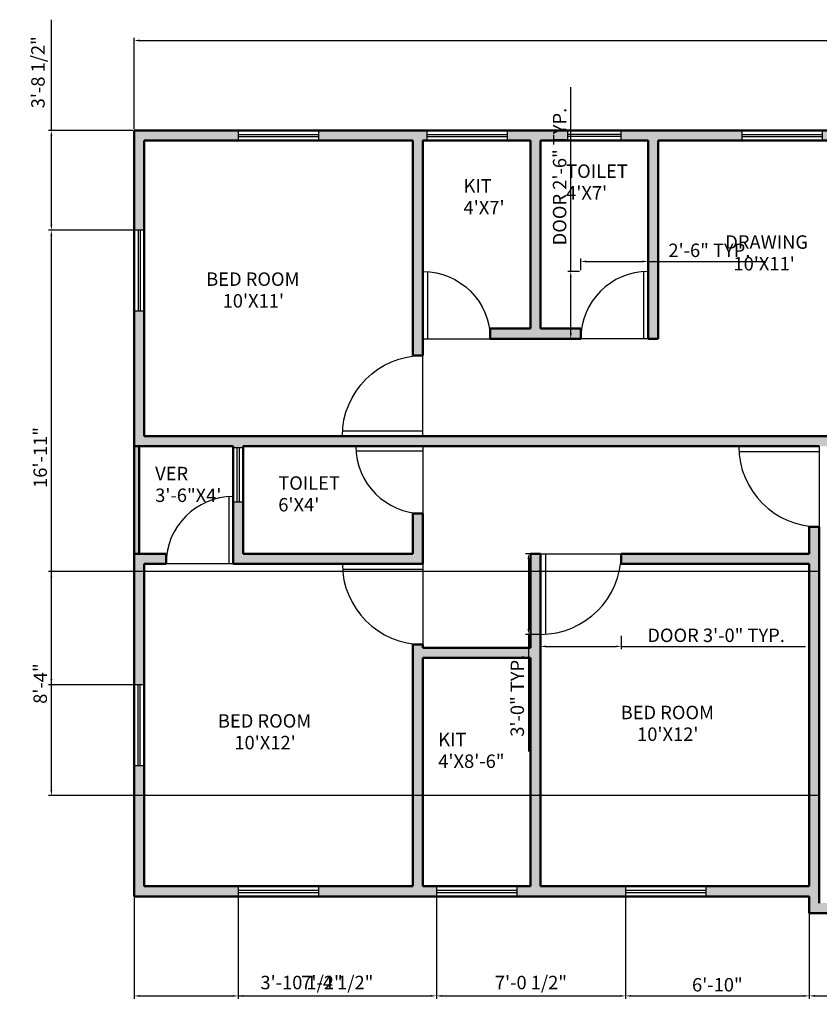
# Model space of a CAD drawing. Units: inches. Extents: x 1931 to 2735, y 1903 to 2370.
# Tile 1 of 2: x 1931 to 2288, y 1903 to 2343. Entities that reach past the tile are written whole.
import ezdxf

# ---------------------------------------------------------------- set-up
doc = ezdxf.new("R2010")
doc.units = ezdxf.units.IN
doc.header["$LTSCALE"] = 0.5
for name, color, linetype, lineweight in [('A-ANNO-DIMS', 93, 'Continuous', 18), ('A-AREA-IDEN', 93, 'Continuous', 25), ('DOORS', 121, 'Continuous', 25), ('WALLS', 231, 'Continuous', 50), ('WINDOWS', 200, 'Continuous', 25)]:
    doc.layers.add(name, color=color, linetype=linetype, lineweight=lineweight)
doc.layers.add('A-WALL-PATT', color=143, linetype='Continuous', lineweight=13, true_color=0x7aafdf)
doc.styles.get("Standard").update_dxf_attribs({"font": 'txt', "height": 6})
doc.dimstyles.new('ISO-25', dxfattribs={"dimtxt": 5, "dimasz": 2.5, "dimexe": 1.25, "dimexo": 0.625, "dimtad": 1, "dimlunit": 3, "dimtxsty": 'Standard', "dimcen": 2.5, "dimadec": 0, "dimazin": 0, "dimtfac": 1, "dimtmove": 0, "dimatfit": 3, "dimfxl": 1, "dimarcsym": 0})

# ---------------------------------------------------------------- blocks, each defined once
blk = doc.blocks.new('*D1')
at = {"layer": 'A-ANNO-DIMS', "color": 0, "lineweight": -2, "transparency": 16777216}
for p, q in [((1982.32, 2294.17), (1982.32, 2334.97)), ((2694.32, 2294.17), (2694.32, 2334.97)), ((1984.82, 2333.72), (2691.82, 2333.72))]:
    blk.add_line(p, q, dxfattribs=at)
at = {"layer": 'A-ANNO-DIMS', "color": 0, "lineweight": 100, "transparency": 16777216}
for points in [[(1984.82, 2334.14), (1984.82, 2333.3), (1982.32, 2333.72)], [(2691.82, 2334.14), (2691.82, 2333.3), (2694.32, 2333.72)]]:
    blk.add_solid(points, dxfattribs=at)
at = {"layer": 'Defpoints', "color": 0, "lineweight": 100, "transparency": 16777216}
for p in [(2694.32, 2333.72), (1982.32, 2293.55), (2694.32, 2293.55)]:
    blk.add_point(p, dxfattribs=at)
at = {"layer": 'A-ANNO-DIMS', "color": 0, "transparency": 16777216, "insert": (2338.32, 2337.92), "char_height": 6, "attachment_point": 5}
blk.add_mtext('59\'-4"', dxfattribs=at)
blk = doc.blocks.new('DOOR-SWING-36IN')
for p, q in [((0, 0), (0, 36)), ((35.92, 2.4), (0, 2.4)), ((36, 0), (0, 0))]:
    blk.add_line(p, q)
blk.add_arc((0, 0), 36, 0, 90)
blk = doc.blocks.new('DOOR-SWING-30IN')
for p, q in [((28, 29.93), (28, 0)), ((30, 30), (30, 0)), ((30, 0), (0, 0))]:
    blk.add_line(p, q)
blk.add_arc((30, 0), 30, 90, 180)
blk = doc.blocks.new('WINDOW-36IN')
for p, q in [((0, 36), (0, 0)), ((4.5, 36), (0, 36)), ((1.75, 36), (1.75, 0)), ((2.75, 36), (2.75, 0)), ((4.5, 0), (4.5, 36)), ((0, 0), (4.5, 0))]:
    blk.add_line(p, q)
blk = doc.blocks.new('WINDOW-24IN')
for p, q in [((24, 4.5), (0, 4.5)), ((0, 4.5), (0, 0)), ((24, 0), (24, 4.5)), ((24, 2.75), (0, 2.75)), ((24, 1.75), (0, 1.75)), ((0, 0), (24, 0))]:
    blk.add_line(p, q)
blk = doc.blocks.new('*D11')
at = {"layer": 'A-ANNO-DIMS', "color": 0, "lineweight": -2, "transparency": 16777216}
for p, q in [((2163.82, 2067.92), (2163.82, 2061.9)), ((2199.82, 2067.92), (2199.82, 2061.9)), ((2166.32, 2063.15), (2197.32, 2063.15)), ((2199.82, 2063.15), (2282.14, 2063.15))]:
    blk.add_line(p, q, dxfattribs=at)
at = {"layer": 'A-ANNO-DIMS', "color": 0, "lineweight": 100, "transparency": 16777216}
for points in [[(2166.32, 2063.56), (2166.32, 2062.73), (2163.82, 2063.15)], [(2197.32, 2063.56), (2197.32, 2062.73), (2199.82, 2063.15)]]:
    blk.add_solid(points, dxfattribs=at)
at = {"layer": 'Defpoints', "color": 0, "lineweight": 100, "transparency": 16777216}
for p in [(2163.82, 2068.55), (2199.82, 2068.55), (2199.82, 2063.15)]:
    blk.add_point(p, dxfattribs=at)
at = {"layer": 'A-ANNO-DIMS', "color": 0, "transparency": 16777216, "insert": (2242.23, 2067.34), "char_height": 6, "attachment_point": 5}
blk.add_mtext('DOOR 3\'-0" TYP.', dxfattribs=at)
blk = doc.blocks.new('*D12')
at = {"layer": 'A-ANNO-DIMS', "color": 0, "lineweight": -2, "transparency": 16777216}
for p, q in [((2163.19, 2104.55), (2157.17, 2104.55)), ((2158.42, 2102.05), (2158.42, 2071.05)), ((2163.19, 2068.55), (2157.17, 2068.55)), ((2158.42, 2068.55), (2158.42, 2016.22))]:
    blk.add_line(p, q, dxfattribs=at)
at = {"layer": 'A-ANNO-DIMS', "color": 0, "lineweight": 100, "transparency": 16777216}
for points in [[(2158, 2102.05), (2158.83, 2102.05), (2158.42, 2104.55)], [(2158, 2071.05), (2158.83, 2071.05), (2158.42, 2068.55)]]:
    blk.add_solid(points, dxfattribs=at)
at = {"layer": 'Defpoints', "color": 0, "lineweight": 100, "transparency": 16777216}
for p in [(2163.82, 2104.55), (2158.42, 2068.55), (2163.82, 2068.55)]:
    blk.add_point(p, dxfattribs=at)
at = {"layer": 'A-ANNO-DIMS', "color": 0, "transparency": 16777216, "insert": (2154.22, 2041.13), "char_height": 6, "attachment_point": 5, "rotation": 90}
blk.add_mtext('3\'-0" TYP.', dxfattribs=at)
blk = doc.blocks.new('*D13')
at = {"layer": 'A-ANNO-DIMS', "color": 0, "lineweight": -2, "transparency": 16777216}
for p, q in [((2177.32, 2230.55), (2177.32, 2312.87)), ((2181.19, 2230.55), (2176.07, 2230.55)), ((2177.32, 2203.05), (2177.32, 2228.05)), ((2181.19, 2200.55), (2176.07, 2200.55))]:
    blk.add_line(p, q, dxfattribs=at)
at = {"layer": 'A-ANNO-DIMS', "color": 0, "lineweight": 100, "transparency": 16777216}
for points in [[(2176.9, 2228.05), (2177.73, 2228.05), (2177.32, 2230.55)], [(2176.9, 2203.05), (2177.73, 2203.05), (2177.32, 2200.55)]]:
    blk.add_solid(points, dxfattribs=at)
at = {"layer": 'Defpoints', "color": 0, "lineweight": 100, "transparency": 16777216}
for p in [(2177.32, 2230.55), (2181.82, 2230.55), (2181.82, 2200.55)]:
    blk.add_point(p, dxfattribs=at)
at = {"layer": 'A-ANNO-DIMS', "color": 0, "transparency": 16777216, "insert": (2173.12, 2272.96), "char_height": 6, "attachment_point": 5, "rotation": 90}
blk.add_mtext('DOOR 2\'-6" TYP.', dxfattribs=at)
blk = doc.blocks.new('*D14')
at = {"layer": 'A-ANNO-DIMS', "color": 0, "lineweight": -2, "transparency": 16777216}
for p, q in [((2181.82, 2231.17), (2181.82, 2236.3)), ((2184.32, 2235.05), (2209.32, 2235.05)), ((2211.82, 2231.17), (2211.82, 2236.3)), ((2211.82, 2235.05), (2264.14, 2235.05))]:
    blk.add_line(p, q, dxfattribs=at)
at = {"layer": 'A-ANNO-DIMS', "color": 0, "lineweight": 100, "transparency": 16777216}
for points in [[(2184.32, 2235.46), (2184.32, 2234.63), (2181.82, 2235.05)], [(2209.32, 2235.46), (2209.32, 2234.63), (2211.82, 2235.05)]]:
    blk.add_solid(points, dxfattribs=at)
at = {"layer": 'Defpoints', "color": 0, "lineweight": 100, "transparency": 16777216}
for p in [(2211.82, 2235.05), (2181.82, 2230.55), (2211.82, 2230.55)]:
    blk.add_point(p, dxfattribs=at)
at = {"layer": 'A-ANNO-DIMS', "color": 0, "transparency": 16777216, "insert": (2239.23, 2239.24), "char_height": 6, "attachment_point": 5}
blk.add_mtext('2\'-6" TYP.', dxfattribs=at)
blk = doc.blocks.new('*D15')
at = {"layer": 'A-ANNO-DIMS', "color": 0, "lineweight": -2, "transparency": 16777216}
for p, q in [((1982.32, 1950.92), (1982.32, 1905.85)), ((2028.82, 1950.92), (2028.82, 1905.85)), ((1984.82, 1907.1), (2026.32, 1907.1)), ((2028.82, 1907.1), (2082.85, 1907.1))]:
    blk.add_line(p, q, dxfattribs=at)
at = {"layer": 'A-ANNO-DIMS', "color": 0, "lineweight": 100, "transparency": 16777216}
for points in [[(1984.82, 1907.51), (1984.82, 1906.68), (1982.32, 1907.1)], [(2026.32, 1907.51), (2026.32, 1906.68), (2028.82, 1907.1)]]:
    blk.add_solid(points, dxfattribs=at)
at = {"layer": 'Defpoints', "color": 0, "lineweight": 100, "transparency": 16777216}
for p in [(1982.32, 1951.55), (2028.82, 1951.55), (2028.82, 1907.1)]:
    blk.add_point(p, dxfattribs=at)
at = {"layer": 'A-ANNO-DIMS', "color": 0, "transparency": 16777216, "insert": (2057.09, 1912.29), "char_height": 6, "attachment_point": 5}
blk.add_mtext('3\'-10 1/2"', dxfattribs=at)
blk = doc.blocks.new('*D16')
at = {"layer": 'A-ANNO-DIMS', "color": 0, "lineweight": -2, "transparency": 16777216}
for p, q in [((2028.82, 1950.92), (2028.82, 1905.85)), ((2117.32, 1950.92), (2117.32, 1905.85)), ((2031.32, 1907.1), (2114.82, 1907.1))]:
    blk.add_line(p, q, dxfattribs=at)
at = {"layer": 'A-ANNO-DIMS', "color": 0, "lineweight": 100, "transparency": 16777216}
for points in [[(2031.32, 1907.51), (2031.32, 1906.68), (2028.82, 1907.1)], [(2114.82, 1907.51), (2114.82, 1906.68), (2117.32, 1907.1)]]:
    blk.add_solid(points, dxfattribs=at)
at = {"layer": 'Defpoints', "color": 0, "lineweight": 100, "transparency": 16777216}
for p in [(2028.82, 1951.55), (2117.32, 1951.55), (2117.32, 1907.1)]:
    blk.add_point(p, dxfattribs=at)
at = {"layer": 'A-ANNO-DIMS', "color": 0, "transparency": 16777216, "insert": (2073.07, 1912.29), "char_height": 6, "attachment_point": 5}
blk.add_mtext('7\'-4 1/2"', dxfattribs=at)
blk = doc.blocks.new('*D17')
at = {"layer": 'A-ANNO-DIMS', "color": 0, "lineweight": -2, "transparency": 16777216}
for p, q in [((2117.32, 1950.92), (2117.32, 1905.85)), ((2201.75, 1950.92), (2201.75, 1905.85)), ((2119.82, 1907.1), (2199.25, 1907.1))]:
    blk.add_line(p, q, dxfattribs=at)
at = {"layer": 'A-ANNO-DIMS', "color": 0, "lineweight": 100, "transparency": 16777216}
for points in [[(2119.82, 1907.51), (2119.82, 1906.68), (2117.32, 1907.1)], [(2199.25, 1907.51), (2199.25, 1906.68), (2201.75, 1907.1)]]:
    blk.add_solid(points, dxfattribs=at)
at = {"layer": 'Defpoints', "color": 0, "lineweight": 100, "transparency": 16777216}
for p in [(2117.32, 1951.55), (2201.75, 1951.55), (2201.75, 1907.1)]:
    blk.add_point(p, dxfattribs=at)
at = {"layer": 'A-ANNO-DIMS', "color": 0, "transparency": 16777216, "insert": (2159.53, 1912.29), "char_height": 6, "attachment_point": 5}
blk.add_mtext('7\'-0 1/2"', dxfattribs=at)
blk = doc.blocks.new('*D18')
at = {"layer": 'A-ANNO-DIMS', "color": 0, "lineweight": -2, "transparency": 16777216}
for p, q in [((2201.75, 1950.92), (2201.75, 1905.85)), ((2283.82, 1950.92), (2283.82, 1905.85)), ((2204.25, 1907.1), (2281.32, 1907.1))]:
    blk.add_line(p, q, dxfattribs=at)
at = {"layer": 'A-ANNO-DIMS', "color": 0, "lineweight": 100, "transparency": 16777216}
for points in [[(2204.25, 1907.51), (2204.25, 1906.68), (2201.75, 1907.1)], [(2281.32, 1907.51), (2281.32, 1906.68), (2283.82, 1907.1)]]:
    blk.add_solid(points, dxfattribs=at)
at = {"layer": 'Defpoints', "color": 0, "lineweight": 100, "transparency": 16777216}
for p in [(2201.75, 1951.55), (2283.82, 1951.55), (2283.82, 1907.1)]:
    blk.add_point(p, dxfattribs=at)
at = {"layer": 'A-ANNO-DIMS', "color": 0, "transparency": 16777216, "insert": (2242.78, 1911.29), "char_height": 6, "attachment_point": 5}
blk.add_mtext('6\'-10"', dxfattribs=at)
blk = doc.blocks.new('*D19')
at = {"layer": 'A-ANNO-DIMS', "color": 0, "lineweight": -2, "transparency": 16777216}
for p, q in [((2283.82, 1943.42), (2283.82, 1905.85)), ((2312.44, 1943.42), (2312.44, 1905.85)), ((2286.32, 1907.1), (2309.94, 1907.1)), ((2312.44, 1907.1), (2361.91, 1907.1))]:
    blk.add_line(p, q, dxfattribs=at)
at = {"layer": 'A-ANNO-DIMS', "color": 0, "lineweight": 100, "transparency": 16777216}
for points in [[(2286.32, 1907.51), (2286.32, 1906.68), (2283.82, 1907.1)], [(2309.94, 1907.51), (2309.94, 1906.68), (2312.44, 1907.1)]]:
    blk.add_solid(points, dxfattribs=at)
at = {"layer": 'Defpoints', "color": 0, "lineweight": 100, "transparency": 16777216}
for p in [(2283.82, 1944.05), (2312.44, 1944.05), (2312.44, 1907.1)]:
    blk.add_point(p, dxfattribs=at)
at = {"layer": 'A-ANNO-DIMS', "color": 0, "transparency": 16777216, "insert": (2338.42, 1912.29), "char_height": 6, "attachment_point": 5}
blk.add_mtext('2\'-4 1/2"', dxfattribs=at)
blk = doc.blocks.new('*D26')
at = {"layer": 'A-ANNO-DIMS', "color": 0, "lineweight": -2, "transparency": 16777216}
for p, q in [((2287.69, 2096.55), (1944.12, 2096.55)), ((1945.37, 1999.05), (1945.37, 2094.05)), ((2287.69, 1996.55), (1944.12, 1996.55))]:
    blk.add_line(p, q, dxfattribs=at)
at = {"layer": 'A-ANNO-DIMS', "color": 0, "lineweight": 100, "transparency": 16777216}
for points in [[(1944.95, 2094.05), (1945.78, 2094.05), (1945.37, 2096.55)], [(1944.95, 1999.05), (1945.78, 1999.05), (1945.37, 1996.55)]]:
    blk.add_solid(points, dxfattribs=at)
at = {"layer": 'Defpoints', "color": 0, "lineweight": 100, "transparency": 16777216}
for p in [(1945.37, 2096.55), (2288.32, 2096.55), (2288.32, 1996.55)]:
    blk.add_point(p, dxfattribs=at)
at = {"layer": 'A-ANNO-DIMS', "color": 0, "transparency": 16777216, "insert": (1941.17, 2046.55), "char_height": 6, "attachment_point": 5, "rotation": 90}
blk.add_mtext('8\'-4"', dxfattribs=at)
blk = doc.blocks.new('*D28')
at = {"layer": 'A-ANNO-DIMS', "color": 0, "lineweight": -2, "transparency": 16777216}
for p, q in [((1945.37, 2293.55), (1945.37, 2343.01)), ((1981.69, 2293.55), (1944.12, 2293.55)), ((1945.37, 2251.5), (1945.37, 2291.05)), ((1981.69, 2249), (1944.12, 2249))]:
    blk.add_line(p, q, dxfattribs=at)
at = {"layer": 'A-ANNO-DIMS', "color": 0, "lineweight": 100, "transparency": 16777216}
for points in [[(1944.95, 2291.05), (1945.78, 2291.05), (1945.37, 2293.55)], [(1944.95, 2251.5), (1945.78, 2251.5), (1945.37, 2249)]]:
    blk.add_solid(points, dxfattribs=at)
at = {"layer": 'Defpoints', "color": 0, "lineweight": 100, "transparency": 16777216}
for p in [(1945.37, 2293.55), (1982.32, 2293.55), (1982.32, 2249)]:
    blk.add_point(p, dxfattribs=at)
at = {"layer": 'A-ANNO-DIMS', "color": 0, "transparency": 16777216, "insert": (1940.17, 2319.53), "char_height": 6, "attachment_point": 5, "rotation": 90}
blk.add_mtext('3\'-8 1/2"', dxfattribs=at)
blk = doc.blocks.new('*D29')
at = {"layer": 'A-ANNO-DIMS', "color": 0, "lineweight": -2, "transparency": 16777216}
for p, q in [((1981.69, 2249), (1944.12, 2249)), ((1945.37, 2048.55), (1945.37, 2246.5)), ((1981.69, 2046.05), (1944.12, 2046.05))]:
    blk.add_line(p, q, dxfattribs=at)
at = {"layer": 'A-ANNO-DIMS', "color": 0, "lineweight": 100, "transparency": 16777216}
for points in [[(1944.95, 2246.5), (1945.78, 2246.5), (1945.37, 2249)], [(1944.95, 2048.55), (1945.78, 2048.55), (1945.37, 2046.05)]]:
    blk.add_solid(points, dxfattribs=at)
at = {"layer": 'Defpoints', "color": 0, "lineweight": 100, "transparency": 16777216}
for p in [(1945.37, 2249), (1982.32, 2249), (1982.32, 2046.05)]:
    blk.add_point(p, dxfattribs=at)
at = {"layer": 'A-ANNO-DIMS', "color": 0, "transparency": 16777216, "insert": (1941.17, 2147.52), "char_height": 6, "attachment_point": 5, "rotation": 90}
blk.add_mtext('16\'-11"', dxfattribs=at)

msp = doc.modelspace()

# ---------------------------------------------------------------- hatches: boundary and pattern name
at = {"layer": 'A-WALL-PATT'}
h = msp.add_hatch(color=256, dxfattribs=at)
h.dxf.hatch_style = 1
h.paths.add_polyline_path([(2028.817, 2293.545), (1982.317, 2293.545), (1982.317, 2249.002), (1986.817, 2249.002), (1986.817, 2289.045), (2028.817, 2289.045)])
h.paths.add_polyline_path([(2113.054, 2293.545), (2064.817, 2293.545), (2064.817, 2289.045), (2106.817, 2289.045), (2106.817, 2193.045), (2111.317, 2193.045), (2111.317, 2200.545), (2111.317, 2230.545), (2111.317, 2289.045), (2113.054, 2289.045)])
h.paths.add_polyline_path([(2175.817, 2293.545), (2149.054, 2293.545), (2149.054, 2289.045), (2159.317, 2289.045), (2159.317, 2205.045), (2141.317, 2205.045), (2141.317, 2200.545), (2181.817, 2200.545), (2181.817, 2205.045), (2163.817, 2205.045), (2163.817, 2289.045), (2175.817, 2289.045)])
h.paths.add_polyline_path([(2253.691, 2293.545), (2199.817, 2293.545), (2199.817, 2289.045), (2211.817, 2289.045), (2211.817, 2200.545), (2216.317, 2200.545), (2216.317, 2289.045), (2253.691, 2289.045)])
h.paths.add_polyline_path([(2377.162, 2293.545), (2289.691, 2293.545), (2289.691, 2289.045), (2336.317, 2289.045), (2336.317, 2152.545), (2340.817, 2152.545), (2340.817, 2188.545), (2340.817, 2289.045), (2377.162, 2289.045)])
h.paths.add_polyline_path([(2477.317, 2293.545), (2413.162, 2293.545), (2413.162, 2289.045), (2460.817, 2289.045), (2460.817, 2200.545), (2465.317, 2200.545), (2465.317, 2230.545), (2465.317, 2289.045), (2477.317, 2289.045)])
h.paths.add_polyline_path([(2518.935, 2293.545), (2501.317, 2293.545), (2501.317, 2289.045), (2513.317, 2289.045), (2513.317, 2205.045), (2495.317, 2205.045), (2495.317, 2200.545), (2535.817, 2200.545), (2535.817, 2205.045), (2517.817, 2205.045), (2517.817, 2289.045), (2518.935, 2289.045)])
h.paths.add_polyline_path([(2612.067, 2293.545), (2554.935, 2293.545), (2554.935, 2289.045), (2565.817, 2289.045), (2565.817, 2200.545), (2565.817, 2193.045), (2570.317, 2193.045), (2570.317, 2289.045), (2612.067, 2289.045)])
h.paths.add_polyline_path([(2694.317, 2293.545), (2648.067, 2293.545), (2648.067, 2289.045), (2689.817, 2289.045), (2689.817, 2249.002), (2694.317, 2249.002)])
h.paths.add_polyline_path([(2694.317, 2213.002), (2689.817, 2213.002), (2689.817, 2157.045), (2565.817, 2157.045), (2376.817, 2157.045), (2376.817, 2152.545), (2388.817, 2152.545), (2424.817, 2152.545), (2565.817, 2152.545), (2645.567, 2152.545), (2645.567, 2150.653), (2650.067, 2150.653), (2650.067, 2152.545), (2694.317, 2152.545)])
h.paths.add_polyline_path([(2694.317, 2152.545), (2692.067, 2152.545), (2692.067, 2104.545), (2694.317, 2104.545)])
h.paths.add_polyline_path([(2694.317, 2104.545), (2680.067, 2104.545), (2680.067, 2100.045), (2689.817, 2100.045), (2689.817, 2047.537), (2694.317, 2047.537)])
h.paths.add_polyline_path([(2650.067, 2126.653), (2645.567, 2126.653), (2645.567, 2104.545), (2570.317, 2104.545), (2570.317, 2122.545), (2565.817, 2122.545), (2565.817, 2100.045), (2601.817, 2100.045), (2650.067, 2100.045)])
h.paths.add_polyline_path([(2570.317, 2064.045), (2565.817, 2064.045), (2565.817, 2062.545), (2565.817, 2032.545), (2565.817, 1956.045), (2559.817, 1956.045), (2559.817, 1951.545), (2612.067, 1951.545), (2612.067, 1956.045), (2570.317, 1956.045)])
h.paths.add_polyline_path([(2694.317, 2011.537), (2689.817, 2011.537), (2689.817, 1956.045), (2648.067, 1956.045), (2648.067, 1951.545), (2694.317, 1951.545)])
h.paths.add_polyline_path([(2435.317, 1956.045), (2393.317, 1956.045), (2393.317, 2100.045), (2477.317, 2100.045), (2477.317, 2104.545), (2393.317, 2104.545), (2393.317, 2116.545), (2388.817, 2116.545), (2388.817, 1948.545), (2348.443, 1948.545), (2348.443, 1944.045), (2393.317, 1944.045), (2393.317, 1951.545), (2435.317, 1951.545)])
h.paths.add_polyline_path([(2523.817, 1956.045), (2517.817, 1956.045), (2517.817, 2058.045), (2535.817, 2058.045), (2535.817, 2062.545), (2517.817, 2062.545), (2517.817, 2104.545), (2513.317, 2104.545), (2513.317, 2068.545), (2513.317, 1956.045), (2471.317, 1956.045), (2471.317, 1951.545), (2523.817, 1951.545)])
h.paths.add_polyline_path([(2288.317, 2116.545), (2283.817, 2116.545), (2283.817, 2104.545), (2199.817, 2104.545), (2199.817, 2100.045), (2283.817, 2100.045), (2283.817, 1956.045), (2237.745, 1956.045), (2237.745, 1951.545), (2283.817, 1951.545), (2283.817, 1944.045), (2312.443, 1944.045), (2312.443, 1948.545), (2288.317, 1948.545)])
h.paths.add_polyline_path([(2163.817, 2104.545), (2159.317, 2104.545), (2159.317, 2062.545), (2111.317, 2062.545), (2111.317, 2064.045), (2106.817, 2064.045), (2106.817, 1956.045), (2064.817, 1956.045), (2064.817, 1951.545), (2117.317, 1951.545), (2117.317, 1956.045), (2111.317, 1956.045), (2111.317, 2058.045), (2159.317, 2058.045), (2159.317, 1956.045), (2153.317, 1956.045), (2153.317, 1951.545), (2201.745, 1951.545), (2201.745, 1956.045), (2163.817, 1956.045)])
h.paths.add_polyline_path([(2031.067, 2127.762), (2026.567, 2127.762), (2026.567, 2100.045), (2111.317, 2100.045), (2111.317, 2122.545), (2106.817, 2122.545), (2106.817, 2104.545), (2031.067, 2104.545)])
h.paths.add_polyline_path([(1996.567, 2104.545), (1982.317, 2104.545), (1982.317, 2046.045), (1986.817, 2046.045), (1986.817, 2100.045), (1996.567, 2100.045)])
h.paths.add_polyline_path([(1986.817, 2010.045), (1982.317, 2010.045), (1982.317, 1951.545), (2028.817, 1951.545), (2028.817, 1956.045), (1986.817, 1956.045)])
h.paths.add_polyline_path([(1984.567, 2152.545), (1982.317, 2152.545), (1982.317, 2104.545), (1984.567, 2104.545)])
h.paths.add_polyline_path([(1986.817, 2213.002), (1982.317, 2213.002), (1982.317, 2152.545), (1984.567, 2152.545), (2026.567, 2152.545), (2026.567, 2151.762), (2031.067, 2151.762), (2031.067, 2152.545), (2111.317, 2152.545), (2288.317, 2152.545), (2300.317, 2152.545), (2300.317, 2157.045), (2111.317, 2157.045), (2075.317, 2157.045), (1986.817, 2157.045)])

# ---------------------------------------------------------------- linework, layer by layer
at = {"layer": 'WALLS'}
for p, q in [((1982.317, 2293.545), (2694.317, 2293.545)), ((1982.317, 1951.545), (1982.317, 2293.545)), ((1986.817, 2289.045), (2106.817, 2289.045)), ((1986.817, 2157.045), (1986.817, 2289.045)), ((2106.817, 2193.045), (2106.817, 2289.045)), ((2111.317, 2200.545), (2111.317, 2289.045)), ((2111.317, 2289.045), (2159.317, 2289.045)), ((2159.317, 2205.045), (2159.317, 2289.045)), ((2159.317, 2205.045), (2159.317, 2289.045)), ((2163.817, 2205.045), (2163.817, 2289.045)), ((2163.817, 2205.045), (2163.817, 2289.045)), ((2163.817, 2289.045), (2211.817, 2289.045)), ((2211.817, 2200.545), (2211.817, 2289.045)), ((2216.317, 2200.545), (2216.317, 2289.045)), ((2216.317, 2289.045), (2336.317, 2289.045)), ((2141.317, 2205.045), (2159.317, 2205.045)), ((2141.317, 2205.045), (2159.317, 2205.045)), ((2141.317, 2200.545), (2141.317, 2205.045)), ((2163.817, 2205.045), (2181.817, 2205.045)), ((2163.817, 2205.045), (2181.817, 2205.045)), ((2181.817, 2200.545), (2181.817, 2205.045)), ((2111.317, 2193.045), (2111.317, 2200.545)), ((2141.317, 2200.545), (2181.817, 2200.545)), ((2141.317, 2200.545), (2181.817, 2200.545)), ((2211.817, 2200.545), (2216.317, 2200.545)), ((2211.817, 2200.545), (2216.317, 2200.545)), ((2106.817, 2193.045), (2111.317, 2193.045)), ((1986.817, 2157.045), (2111.317, 2157.045)), ((2111.317, 2157.045), (2300.317, 2157.045)), ((1982.317, 2152.545), (2026.567, 2152.545)), ((1984.567, 2104.545), (1984.567, 2152.545)), ((2026.567, 2100.045), (2026.567, 2152.545)), ((2031.067, 2104.545), (2031.067, 2152.545)), ((2031.067, 2152.545), (2111.317, 2152.545)), ((2111.317, 2152.545), (2288.317, 2152.545)), ((2106.817, 2104.545), (2106.817, 2122.545)), ((2106.817, 2122.545), (2111.317, 2122.545)), ((2111.317, 2100.045), (2111.317, 2122.545)), ((2283.817, 2104.545), (2283.817, 2116.545)), ((2283.817, 2116.545), (2288.317, 2116.545)), ((2288.317, 1948.545), (2288.317, 2116.545)), ((1982.317, 2104.545), (1996.567, 2104.545)), ((1996.567, 2100.045), (1996.567, 2104.545)), ((2031.067, 2104.545), (2106.817, 2104.545)), ((2159.317, 2104.545), (2163.817, 2104.545)), ((2159.317, 2062.545), (2159.317, 2104.545)), ((2163.817, 1956.045), (2163.817, 2104.545)), ((2199.817, 2100.045), (2199.817, 2104.545)), ((2199.817, 2104.545), (2283.817, 2104.545)), ((1986.817, 1956.045), (1986.817, 2100.045)), ((1986.817, 2100.045), (1996.567, 2100.045)), ((2026.567, 2100.045), (2111.317, 2100.045)), ((2199.817, 2100.045), (2283.817, 2100.045)), ((2283.817, 1956.045), (2283.817, 2100.045)), ((2106.817, 1956.045), (2106.817, 2064.045)), ((2106.817, 2064.045), (2111.317, 2064.045)), ((2111.317, 2062.545), (2111.317, 2064.045)), ((2159.317, 2062.545), (2111.317, 2062.545)), ((2111.317, 1956.045), (2111.317, 2058.045)), ((2159.317, 2058.045), (2111.317, 2058.045)), ((2159.317, 1956.045), (2159.317, 2058.045)), ((2106.817, 1956.045), (1986.817, 1956.045)), ((2159.317, 1956.045), (2111.317, 1956.045)), ((2283.817, 1956.045), (2163.817, 1956.045)), ((2283.817, 1951.545), (1982.317, 1951.545)), ((2283.817, 1944.045), (2283.817, 1951.545)), ((2283.817, 1944.045), (2393.317, 1944.045))]:
    msp.add_line(p, q, dxfattribs=at)

# ---------------------------------------------------------------- block references
at = {"layer": 'DOORS', "extrusion": (0, 0, -1), "zscale": -1}
for name, p in [('DOOR-SWING-30IN', (-2141.318, 2200.545)), ('DOOR-SWING-36IN', (-2111.318, 2157.045))]:
    msp.add_blockref(name, p, dxfattribs=at)
at = {"layer": 'DOORS'}
for p in [(2181.817, 2200.545), (1996.567, 2100.045)]:
    msp.add_blockref('DOOR-SWING-30IN', p, dxfattribs=at)
for name, p, rotation in [('DOOR-SWING-30IN', (2111.318, 2122.545), 89.9999999999985), ('DOOR-SWING-36IN', (2288.318, 2152.545), 180), ('DOOR-SWING-36IN', (2163.817, 2104.546), 270.0000000000151), ('DOOR-SWING-36IN', (2111.318, 2100.045), 180)]:
    msp.add_blockref(name, p, dxfattribs=dict(at, rotation=rotation))
at = {"layer": 'WINDOWS'}
for name, p, rotation in [('WINDOW-36IN', (2064.818, 2289.045), 90.00000000000072), ('WINDOW-36IN', (2149.054, 2289.045), 90.00000000000018), ('WINDOW-36IN', (2289.691, 2289.045), 90.00000000000072), ('WINDOW-24IN', (2026.567, 2151.763), 270.0000000000041), ('WINDOW-36IN', (1986.818, 2046.045), 180), ('WINDOW-36IN', (2064.818, 1951.545), 90.00000000000144), ('WINDOW-36IN', (2153.318, 1951.545), 90.00000000000144), ('WINDOW-36IN', (2237.746, 1951.545), 90.00000000000144)]:
    msp.add_blockref(name, p, dxfattribs=dict(at, rotation=rotation))
for name, p in [('WINDOW-24IN', (2175.817, 2289.045)), ('WINDOW-36IN', (1982.317, 2213.002))]:
    msp.add_blockref(name, p, dxfattribs=at)

# ---------------------------------------------------------------- texts
at = {"layer": 'A-AREA-IDEN'}
for s, p in [('TOILET', (2175.255, 2272.372)), ('KIT', (2129.439, 2265.818)), ("4'X7'", (2175.255, 2262.673)), ("4'X7'", (2129.439, 2256.12)), ('DRAWING', (2246.313, 2240.729)), ("  10'X11'", (2246.313, 2231.031)), ('BED ROOM', (2014.515, 2224.159)), ("    10'X11'", (2014.515, 2214.461)), ('VER', (1991.726, 2137.348)), ('TOILET', (2046.701, 2133.115)), ('3\'-6"X4\'', (1991.726, 2127.65)), ("6'X4'", (2046.701, 2123.417)), ('BED ROOM', (2199.609, 2030.648)), ('BED ROOM', (2019.756, 2026.899)), ("    10'X12'", (2199.609, 2020.95)), ("    10'X12'", (2019.756, 2017.201)), ('KIT ', (2118.151, 2018.6)), ('4\'X8\'-6"', (2118.151, 2008.902))]:
    msp.add_text(s, height=6, dxfattribs=at).set_placement(p)

# ---------------------------------------------------------------- dimensions: what is measured, and where the dimension line sits
at = {"layer": 'A-ANNO-DIMS'}
for base, p1, p2, picture, middle in [((1945.367, 2293.545), (1982.317, 2249.002), (1982.317, 2293.545), '*D28', (1940.171, 2319.527)), ((1945.367, 2249.002), (1982.317, 2046.045), (1982.317, 2249.002), '*D29', (1941.171, 2147.524)), ((1945.367, 2096.545), (2288.317, 1996.545), (2288.317, 2096.545), '*D26', (1941.171, 2046.545))]:
    dim = msp.add_linear_dim(base=base, p1=p1, p2=p2, angle=90, dimstyle='ISO-25', override={"dimdec": 1, "dimlfac": 1, "dimrnd": 0, "dimzin": 1, "dimdsep": 46, "dimlunit": 4, "dimfrac": 2}, dxfattribs=at)
    dim.commit()
    dim.dimension.update_dxf_attribs({"geometry": picture, "text_midpoint": middle})
for base, p1, p2, override, picture, middle in [((2694.317, 2333.721), (1982.317, 2293.545), (2694.317, 2293.545), {"dimclrd": 0, "dimclre": 0, "dimclrt": 0}, '*D1', (2338.317, 2337.918)), ((2028.817, 1907.095), (1982.317, 1951.545), (2028.817, 1951.545), {"dimdec": 1, "dimlfac": 1, "dimrnd": 0, "dimzin": 1, "dimdsep": 46, "dimlunit": 4, "dimfrac": 2}, '*D15', (2057.085, 1912.292)), ((2117.317, 1907.095), (2028.817, 1951.545), (2117.317, 1951.545), {"dimdec": 1, "dimlfac": 1, "dimrnd": 0, "dimzin": 1, "dimdsep": 46, "dimlunit": 4, "dimfrac": 2}, '*D16', (2073.067, 1912.292)), ((2201.745, 1907.095), (2117.317, 1951.545), (2201.745, 1951.545), {"dimdec": 1, "dimlfac": 1, "dimrnd": 0, "dimzin": 1, "dimdsep": 46, "dimlunit": 4, "dimfrac": 2}, '*D17', (2159.531, 1912.292)), ((2283.817, 1907.095), (2201.745, 1951.545), (2283.817, 1951.545), {"dimdec": 1, "dimlfac": 1, "dimrnd": 0, "dimzin": 1, "dimdsep": 46, "dimlunit": 4, "dimfrac": 2}, '*D18', (2242.781, 1911.292)), ((2312.443, 1907.095), (2283.817, 1944.045), (2312.443, 1944.045), {"dimdec": 1, "dimlfac": 1, "dimrnd": 0, "dimzin": 1, "dimdsep": 46, "dimlunit": 4, "dimfrac": 2}, '*D19', (2338.425, 1912.292))]:
    dim = msp.add_linear_dim(base=base, p1=p1, p2=p2, dimstyle='ISO-25', override=override, dxfattribs=at)
    dim.commit()
    dim.dimension.update_dxf_attribs({"geometry": picture, "text_midpoint": middle})
for base, p1, p2, angle, text, picture, middle in [((2177.317, 2230.545), (2181.817, 2200.545), (2181.817, 2230.545), 90, 'DOOR <> TYP.', '*D13', (2173.121, 2272.956)), ((2158.417, 2068.545), (2163.817, 2104.545), (2163.817, 2068.545), 270, '<> TYP.', '*D12', (2154.221, 2041.134)), ((2199.817, 2063.145), (2163.817, 2068.545), (2199.817, 2068.545), 0, 'DOOR <> TYP.', '*D11', (2242.228, 2067.342))]:
    dim = msp.add_linear_dim(base=base, p1=p1, p2=p2, angle=angle, text=text, dimstyle='ISO-25', override={"dimdec": 1, "dimlfac": 1, "dimrnd": 0, "dimzin": 1, "dimdsep": 46, "dimlunit": 4, "dimfrac": 2}, dxfattribs=at)
    dim.commit()
    dim.dimension.update_dxf_attribs({"geometry": picture, "text_midpoint": middle})
dim = msp.add_linear_dim(base=(2211.817, 2235.045), p1=(2181.817, 2230.545), p2=(2211.817, 2230.545), text='<> TYP.', dimstyle='ISO-25', override={"dimdec": 1, "dimlfac": 1, "dimrnd": 0, "dimzin": 1, "dimdsep": 46, "dimlunit": 4, "dimfrac": 2}, dxfattribs=at)
dim.commit()
dim.dimension.update_dxf_attribs({"geometry": '*D14', "text_midpoint": (2239.228, 2239.242)})

doc.saveas('drawing.dxf')
